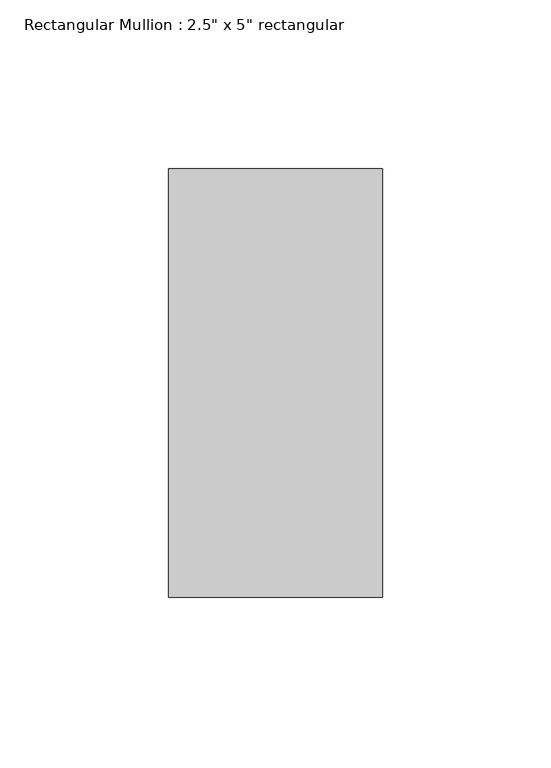
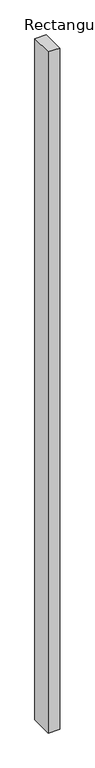
"""IFC4 building model written with IfcOpenShell, lengths in millimetres: member geometry."""

from ifc_helpers import new_model, si_unit, frame, origin, place, context, project, spatial, polyline, outline, extrude, source, transform, mapped, element, save


def member_ab6d823a(model_context):
    return source(origin(), model_context, "Body", "SweptSolid", [
        extrude(outline(polyline([(0.0, 63.5), (0.0, -63.5), (-63.5, -63.5), (-63.5, 63.5), (0.0, 63.5)])), frame((0.0, 0.0, -3958.2450638), z_axis=(0.0, 0.0, 1.0), x_axis=(1.0, 0.0, 0.0)), (0.0, 0.0, 1.0), 3958.2450638),
    ])


if __name__ == "__main__":
    model = new_model("IFC4")
    model_context = context("Model", 3, world=origin())
    ifc_project = project(units=[si_unit("LENGTHUNIT", "METRE", prefix="MILLI")], contexts=[model_context])
    site = spatial("IfcSite", under=ifc_project)
    building = spatial("IfcBuilding", under=site)
    placement = place(None, origin())
    member_shape = member_ab6d823a(model_context)
    element("IfcMember", 1, ObjectType="Rectangular Mullion : 2.5\" x 5\" rectangular", at=placement, inside=building, context=model_context, shape_type="MappedRepresentation", body=[
        mapped(member_shape, transform((0.0, 0.0, 0.0), x_axis=(1.0, 0.0, 0.0), y_axis=(0.0, 1.0, 0.0), z_axis=(0.0, 0.0, 1.0))),
    ])
    save(model, "model.ifc")

# Revit data of these elements
# Type "Rectangular Mullion : 2.5\" x 5\" rectangular"
#   built-in parameter 1007304 = 0.416667 (stored number, unit not read)
#   built-in parameter 1007301 = 0.104167 (stored number, unit not read)
#   built-in parameter 1007300 = 0.104167 (stored number, unit not read)
# Element 1 (IfcMember, "Rectangular Mullion : 2.5\" x 5\" rectangular")
#   Materials on its faces: "Aluminum"
# Materials
#   "Aluminum": class "Metal", colour RGB 247 247 247, transparency 0, Description = "Aluminum 6061", Cost = 0
